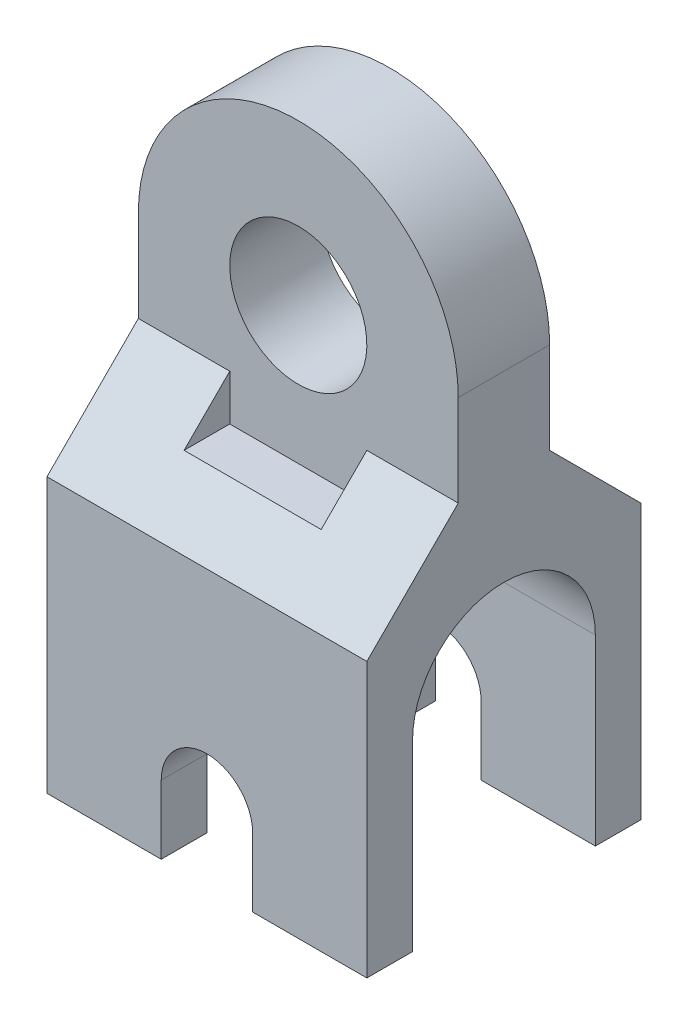
ISO-10303-21;
HEADER;
FILE_DESCRIPTION(('STEP AP214'),'2;1');
FILE_NAME('part.step','',(''),(''),'','','');
FILE_SCHEMA(('AUTOMOTIVE_DESIGN { 1 0 10303 214 1 1 1 1 }'));
ENDSEC;
DATA;
#1=APPLICATION_CONTEXT('core data for automotive mechanical design processes');
#2=APPLICATION_PROTOCOL_DEFINITION('international standard','automotive_design',2000,#1);
#3=PRODUCT_CONTEXT('',#1,'mechanical');
#4=PRODUCT('Part','Part','',(#3));
#5=PRODUCT_RELATED_PRODUCT_CATEGORY('part','',(#4));
#6=PRODUCT_DEFINITION_FORMATION('','',#4);
#7=PRODUCT_DEFINITION_CONTEXT('part definition',#1,'design');
#8=PRODUCT_DEFINITION('design','',#6,#7);
#9=PRODUCT_DEFINITION_SHAPE('','',#8);
#10=(LENGTH_UNIT() NAMED_UNIT(*) SI_UNIT(.MILLI.,.METRE.));
#11=(NAMED_UNIT(*) PLANE_ANGLE_UNIT() SI_UNIT($,.RADIAN.));
#12=(NAMED_UNIT(*) SI_UNIT($,.STERADIAN.) SOLID_ANGLE_UNIT());
#13=UNCERTAINTY_MEASURE_WITH_UNIT(LENGTH_MEASURE(1.E-05),#10,'distance_accuracy_value','');
#14=(GEOMETRIC_REPRESENTATION_CONTEXT(3) GLOBAL_UNCERTAINTY_ASSIGNED_CONTEXT((#13)) GLOBAL_UNIT_ASSIGNED_CONTEXT((#10,
#11,#12)) REPRESENTATION_CONTEXT('',''));
#15=CARTESIAN_POINT('',(0.,0.,0.));
#16=DIRECTION('',(0.,0.,1.));
#17=DIRECTION('',(1.,0.,0.));
#18=AXIS2_PLACEMENT_3D('',#15,#16,#17);
#19=CARTESIAN_POINT('',(35.,0.,30.));
#20=DIRECTION('',(0.,-0.707106781186548,-0.707106781186548));
#21=DIRECTION('',(0.,0.707106781186548,-0.707106781186548));
#22=AXIS2_PLACEMENT_3D('',#19,#20,#21);
#23=PLANE('',#22);
#24=DIRECTION('',(0.,-0.707106781186548,0.707106781186548));
#25=VECTOR('',#24,1.);
#26=CARTESIAN_POINT('',(-15.,0.,30.));
#27=LINE('',#26,#25);
#28=CARTESIAN_POINT('',(-15.,20.,10.));
#29=VERTEX_POINT('',#28);
#30=CARTESIAN_POINT('',(-15.,10.,20.));
#31=VERTEX_POINT('',#30);
#32=EDGE_CURVE('E11',#29,#31,#27,.T.);
#33=ORIENTED_EDGE('',*,*,#32,.F.);
#34=DIRECTION('',(-1.,0.,0.));
#35=VECTOR('',#34,1.);
#36=CARTESIAN_POINT('',(35.,20.,10.));
#37=LINE('',#36,#35);
#38=CARTESIAN_POINT('',(-35.,20.,10.));
#39=VERTEX_POINT('',#38);
#40=EDGE_CURVE('E367',#29,#39,#37,.T.);
#41=ORIENTED_EDGE('',*,*,#40,.T.);
#42=DIRECTION('',(0.,-0.707106781186548,0.707106781186548));
#43=VECTOR('',#42,1.);
#44=CARTESIAN_POINT('',(-35.,0.,30.));
#45=LINE('',#44,#43);
#46=CARTESIAN_POINT('',(-35.,0.,30.));
#47=VERTEX_POINT('',#46);
#48=EDGE_CURVE('E316',#39,#47,#45,.T.);
#49=ORIENTED_EDGE('',*,*,#48,.T.);
#50=DIRECTION('',(-1.,0.,0.));
#51=VECTOR('',#50,1.);
#52=CARTESIAN_POINT('',(35.,0.,30.));
#53=LINE('',#52,#51);
#54=CARTESIAN_POINT('',(35.,0.,30.));
#55=VERTEX_POINT('',#54);
#56=EDGE_CURVE('E337',#55,#47,#53,.T.);
#57=ORIENTED_EDGE('',*,*,#56,.F.);
#58=DIRECTION('',(0.,-0.707106781186548,0.707106781186548));
#59=VECTOR('',#58,1.);
#60=CARTESIAN_POINT('',(35.,0.,30.));
#61=LINE('',#60,#59);
#62=CARTESIAN_POINT('',(35.,20.,10.));
#63=VERTEX_POINT('',#62);
#64=EDGE_CURVE('E338',#63,#55,#61,.T.);
#65=ORIENTED_EDGE('',*,*,#64,.F.);
#66=CARTESIAN_POINT('',(15.,20.,10.));
#67=VERTEX_POINT('',#66);
#68=EDGE_CURVE('E371',#63,#67,#37,.T.);
#69=ORIENTED_EDGE('',*,*,#68,.T.);
#70=DIRECTION('',(0.,0.707106781186548,-0.707106781186548));
#71=VECTOR('',#70,1.);
#72=CARTESIAN_POINT('',(15.,0.,30.));
#73=LINE('',#72,#71);
#74=CARTESIAN_POINT('',(15.,10.,20.));
#75=VERTEX_POINT('',#74);
#76=EDGE_CURVE('E47',#75,#67,#73,.T.);
#77=ORIENTED_EDGE('',*,*,#76,.F.);
#78=DIRECTION('',(-1.,0.,0.));
#79=VECTOR('',#78,1.);
#80=CARTESIAN_POINT('',(-15.,10.,20.));
#81=LINE('',#80,#79);
#82=EDGE_CURVE('E228',#75,#31,#81,.T.);
#83=ORIENTED_EDGE('',*,*,#82,.T.);
#84=EDGE_LOOP('',(#33,#41,#49,#57,#65,#69,#77,#83));
#85=FACE_BOUND('',#84,.T.);
#86=ADVANCED_FACE('F41',(#85),#23,.F.);
#87=CARTESIAN_POINT('',(35.,-60.,30.));
#88=DIRECTION('',(0.,1.,0.));
#89=DIRECTION('',(0.,0.,1.));
#90=AXIS2_PLACEMENT_3D('',#87,#88,#89);
#91=PLANE('',#90);
#92=DIRECTION('',(-1.,0.,0.));
#93=VECTOR('',#92,1.);
#94=CARTESIAN_POINT('',(35.,-60.,20.));
#95=LINE('',#94,#93);
#96=CARTESIAN_POINT('',(-10.,-60.,20.));
#97=VERTEX_POINT('',#96);
#98=CARTESIAN_POINT('',(-35.,-60.,20.));
#99=VERTEX_POINT('',#98);
#100=EDGE_CURVE('E395',#97,#99,#95,.T.);
#101=ORIENTED_EDGE('',*,*,#100,.F.);
#102=DIRECTION('',(0.,0.,-1.));
#103=VECTOR('',#102,1.);
#104=CARTESIAN_POINT('',(-10.,-60.,30.0000000000001));
#105=LINE('',#104,#103);
#106=CARTESIAN_POINT('',(-10.,-60.,30.0000000000001));
#107=VERTEX_POINT('',#106);
#108=EDGE_CURVE('E274',#107,#97,#105,.T.);
#109=ORIENTED_EDGE('',*,*,#108,.F.);
#110=DIRECTION('',(-1.,0.,0.));
#111=VECTOR('',#110,1.);
#112=CARTESIAN_POINT('',(35.,-60.,30.));
#113=LINE('',#112,#111);
#114=CARTESIAN_POINT('',(-35.,-60.,30.));
#115=VERTEX_POINT('',#114);
#116=EDGE_CURVE('E400',#107,#115,#113,.T.);
#117=ORIENTED_EDGE('',*,*,#116,.T.);
#118=DIRECTION('',(0.,0.,-1.));
#119=VECTOR('',#118,1.);
#120=CARTESIAN_POINT('',(-35.,-60.,30.));
#121=LINE('',#120,#119);
#122=EDGE_CURVE('E342',#115,#99,#121,.T.);
#123=ORIENTED_EDGE('',*,*,#122,.T.);
#124=EDGE_LOOP('',(#101,#109,#117,#123));
#125=FACE_BOUND('',#124,.T.);
#126=ADVANCED_FACE('F440',(#125),#91,.F.);
#127=CARTESIAN_POINT('',(35.,-60.,-20.));
#128=DIRECTION('',(0.,1.,0.));
#129=DIRECTION('',(0.,0.,1.));
#130=AXIS2_PLACEMENT_3D('',#127,#128,#129);
#131=PLANE('',#130);
#132=DIRECTION('',(-1.,0.,0.));
#133=VECTOR('',#132,1.);
#134=CARTESIAN_POINT('',(35.,-60.,-30.));
#135=LINE('',#134,#133);
#136=CARTESIAN_POINT('',(-10.,-60.,-30.));
#137=VERTEX_POINT('',#136);
#138=CARTESIAN_POINT('',(-35.,-60.,-30.));
#139=VERTEX_POINT('',#138);
#140=EDGE_CURVE('E379',#137,#139,#135,.T.);
#141=ORIENTED_EDGE('',*,*,#140,.F.);
#142=CARTESIAN_POINT('',(-10.,-60.,-20.));
#143=VERTEX_POINT('',#142);
#144=EDGE_CURVE('E280',#143,#137,#105,.T.);
#145=ORIENTED_EDGE('',*,*,#144,.F.);
#146=DIRECTION('',(-1.,0.,0.));
#147=VECTOR('',#146,1.);
#148=CARTESIAN_POINT('',(35.,-60.,-20.));
#149=LINE('',#148,#147);
#150=CARTESIAN_POINT('',(-35.,-60.,-20.));
#151=VERTEX_POINT('',#150);
#152=EDGE_CURVE('E383',#143,#151,#149,.T.);
#153=ORIENTED_EDGE('',*,*,#152,.T.);
#154=DIRECTION('',(0.,0.,-1.));
#155=VECTOR('',#154,1.);
#156=CARTESIAN_POINT('',(-35.,-60.,-20.));
#157=LINE('',#156,#155);
#158=EDGE_CURVE('E353',#151,#139,#157,.T.);
#159=ORIENTED_EDGE('',*,*,#158,.T.);
#160=EDGE_LOOP('',(#141,#145,#153,#159));
#161=FACE_BOUND('',#160,.T.);
#162=ADVANCED_FACE('F473',(#161),#131,.F.);
#163=CARTESIAN_POINT('',(35.,0.,30.));
#164=DIRECTION('',(0.,0.,-1.));
#165=DIRECTION('',(0.,1.,0.));
#166=AXIS2_PLACEMENT_3D('',#163,#164,#165);
#167=PLANE('',#166);
#168=ORIENTED_EDGE('',*,*,#116,.F.);
#169=DIRECTION('',(0.,1.,0.));
#170=VECTOR('',#169,1.);
#171=CARTESIAN_POINT('',(-10.,-45.,30.0000000000001));
#172=LINE('',#171,#170);
#173=CARTESIAN_POINT('',(-10.,-45.,30.0000000000001));
#174=VERTEX_POINT('',#173);
#175=EDGE_CURVE('E266',#107,#174,#172,.T.);
#176=ORIENTED_EDGE('',*,*,#175,.T.);
#177=CARTESIAN_POINT('',(0.,-45.,30.0000000000001));
#178=DIRECTION('',(0.,0.,-1.));
#179=DIRECTION('',(0.,1.,0.));
#180=AXIS2_PLACEMENT_3D('',#177,#178,#179);
#181=CIRCLE('',#180,10.);
#182=CARTESIAN_POINT('',(10.,-45.,30.0000000000001));
#183=VERTEX_POINT('',#182);
#184=EDGE_CURVE('E257',#174,#183,#181,.T.);
#185=ORIENTED_EDGE('',*,*,#184,.T.);
#186=DIRECTION('',(0.,-1.,0.));
#187=VECTOR('',#186,1.);
#188=CARTESIAN_POINT('',(10.,-45.,30.0000000000001));
#189=LINE('',#188,#187);
#190=CARTESIAN_POINT('',(10.,-60.,30.0000000000001));
#191=VERTEX_POINT('',#190);
#192=EDGE_CURVE('E263',#183,#191,#189,.T.);
#193=ORIENTED_EDGE('',*,*,#192,.T.);
#194=CARTESIAN_POINT('',(35.,-60.,30.));
#195=VERTEX_POINT('',#194);
#196=EDGE_CURVE('E396',#195,#191,#113,.T.);
#197=ORIENTED_EDGE('',*,*,#196,.F.);
#198=DIRECTION('',(0.,-1.,0.));
#199=VECTOR('',#198,1.);
#200=CARTESIAN_POINT('',(35.,0.,30.));
#201=LINE('',#200,#199);
#202=EDGE_CURVE('E315',#55,#195,#201,.T.);
#203=ORIENTED_EDGE('',*,*,#202,.F.);
#204=ORIENTED_EDGE('',*,*,#56,.T.);
#205=DIRECTION('',(0.,-1.,0.));
#206=VECTOR('',#205,1.);
#207=CARTESIAN_POINT('',(-35.,0.,30.));
#208=LINE('',#207,#206);
#209=EDGE_CURVE('E310',#47,#115,#208,.T.);
#210=ORIENTED_EDGE('',*,*,#209,.T.);
#211=EDGE_LOOP('',(#168,#176,#185,#193,#197,#203,#204,#210));
#212=FACE_BOUND('',#211,.T.);
#213=ADVANCED_FACE('F43',(#212),#167,.F.);
#214=ORIENTED_EDGE('',*,*,#196,.T.);
#215=DIRECTION('',(0.,0.,-1.));
#216=VECTOR('',#215,1.);
#217=CARTESIAN_POINT('',(10.,-60.,30.0000000000001));
#218=LINE('',#217,#216);
#219=CARTESIAN_POINT('',(10.,-60.,20.));
#220=VERTEX_POINT('',#219);
#221=EDGE_CURVE('E279',#191,#220,#218,.T.);
#222=ORIENTED_EDGE('',*,*,#221,.T.);
#223=CARTESIAN_POINT('',(35.,-60.,20.));
#224=VERTEX_POINT('',#223);
#225=EDGE_CURVE('E391',#224,#220,#95,.T.);
#226=ORIENTED_EDGE('',*,*,#225,.F.);
#227=DIRECTION('',(0.,0.,-1.));
#228=VECTOR('',#227,1.);
#229=CARTESIAN_POINT('',(35.,-60.,30.));
#230=LINE('',#229,#228);
#231=EDGE_CURVE('E312',#195,#224,#230,.T.);
#232=ORIENTED_EDGE('',*,*,#231,.F.);
#233=EDGE_LOOP('',(#214,#222,#226,#232));
#234=FACE_BOUND('',#233,.T.);
#235=ADVANCED_FACE('F450',(#234),#91,.F.);
#236=CARTESIAN_POINT('',(35.,-60.,20.));
#237=DIRECTION('',(0.,0.,1.));
#238=DIRECTION('',(0.,-1.,0.));
#239=AXIS2_PLACEMENT_3D('',#236,#237,#238);
#240=PLANE('',#239);
#241=CARTESIAN_POINT('',(0.,-45.,20.));
#242=DIRECTION('',(0.,0.,1.));
#243=DIRECTION('',(0.,-1.,0.));
#244=AXIS2_PLACEMENT_3D('',#241,#242,#243);
#245=CIRCLE('',#244,10.);
#246=CARTESIAN_POINT('',(10.,-45.,20.));
#247=VERTEX_POINT('',#246);
#248=CARTESIAN_POINT('',(-10.,-45.,20.));
#249=VERTEX_POINT('',#248);
#250=EDGE_CURVE('E304',#247,#249,#245,.T.);
#251=ORIENTED_EDGE('',*,*,#250,.T.);
#252=DIRECTION('',(0.,-1.,0.));
#253=VECTOR('',#252,1.);
#254=CARTESIAN_POINT('',(-10.,-60.,20.));
#255=LINE('',#254,#253);
#256=EDGE_CURVE('E298',#249,#97,#255,.T.);
#257=ORIENTED_EDGE('',*,*,#256,.T.);
#258=ORIENTED_EDGE('',*,*,#100,.T.);
#259=DIRECTION('',(0.,1.,0.));
#260=VECTOR('',#259,1.);
#261=CARTESIAN_POINT('',(-35.,-60.,20.));
#262=LINE('',#261,#260);
#263=CARTESIAN_POINT('',(-35.,-20.,20.));
#264=VERTEX_POINT('',#263);
#265=EDGE_CURVE('E341',#99,#264,#262,.T.);
#266=ORIENTED_EDGE('',*,*,#265,.T.);
#267=DIRECTION('',(-1.,0.,0.));
#268=VECTOR('',#267,1.);
#269=CARTESIAN_POINT('',(35.,-20.,20.));
#270=LINE('',#269,#268);
#271=CARTESIAN_POINT('',(35.,-20.,20.));
#272=VERTEX_POINT('',#271);
#273=EDGE_CURVE('E393',#272,#264,#270,.T.);
#274=ORIENTED_EDGE('',*,*,#273,.F.);
#275=DIRECTION('',(0.,1.,0.));
#276=VECTOR('',#275,1.);
#277=CARTESIAN_POINT('',(35.,-60.,20.));
#278=LINE('',#277,#276);
#279=EDGE_CURVE('E318',#224,#272,#278,.T.);
#280=ORIENTED_EDGE('',*,*,#279,.F.);
#281=ORIENTED_EDGE('',*,*,#225,.T.);
#282=DIRECTION('',(0.,1.,0.));
#283=VECTOR('',#282,1.);
#284=CARTESIAN_POINT('',(10.,-60.,20.));
#285=LINE('',#284,#283);
#286=EDGE_CURVE('E288',#220,#247,#285,.T.);
#287=ORIENTED_EDGE('',*,*,#286,.T.);
#288=EDGE_LOOP('',(#251,#257,#258,#266,#274,#280,#281,#287));
#289=FACE_BOUND('',#288,.T.);
#290=ADVANCED_FACE('F493',(#289),#240,.F.);
#291=CARTESIAN_POINT('',(35.,-20.,0.));
#292=DIRECTION('',(-1.,0.,0.));
#293=DIRECTION('',(0.,0.,1.));
#294=AXIS2_PLACEMENT_3D('',#291,#292,#293);
#295=CYLINDRICAL_SURFACE('',#294,20.);
#296=CARTESIAN_POINT('',(-35.,-20.,0.));
#297=DIRECTION('',(-1.,0.,0.));
#298=DIRECTION('',(0.,0.,1.));
#299=AXIS2_PLACEMENT_3D('',#296,#297,#298);
#300=CIRCLE('',#299,20.);
#301=CARTESIAN_POINT('',(-35.,-20.,-20.));
#302=VERTEX_POINT('',#301);
#303=EDGE_CURVE('E347',#264,#302,#300,.T.);
#304=ORIENTED_EDGE('',*,*,#303,.T.);
#305=DIRECTION('',(-1.,0.,0.));
#306=VECTOR('',#305,1.);
#307=CARTESIAN_POINT('',(35.,-20.,-20.));
#308=LINE('',#307,#306);
#309=CARTESIAN_POINT('',(35.,-20.,-20.));
#310=VERTEX_POINT('',#309);
#311=EDGE_CURVE('E389',#310,#302,#308,.T.);
#312=ORIENTED_EDGE('',*,*,#311,.F.);
#313=CARTESIAN_POINT('',(35.,-20.,0.));
#314=DIRECTION('',(-1.,0.,0.));
#315=DIRECTION('',(0.,0.,1.));
#316=AXIS2_PLACEMENT_3D('',#313,#314,#315);
#317=CIRCLE('',#316,20.);
#318=EDGE_CURVE('E319',#272,#310,#317,.T.);
#319=ORIENTED_EDGE('',*,*,#318,.F.);
#320=ORIENTED_EDGE('',*,*,#273,.T.);
#321=EDGE_LOOP('',(#304,#312,#319,#320));
#322=FACE_BOUND('',#321,.T.);
#323=ADVANCED_FACE('F491',(#322),#295,.F.);
#324=CARTESIAN_POINT('',(35.,-20.,-20.));
#325=DIRECTION('',(0.,0.,-1.));
#326=DIRECTION('',(-1.,0.,0.));
#327=AXIS2_PLACEMENT_3D('',#324,#325,#326);
#328=PLANE('',#327);
#329=ORIENTED_EDGE('',*,*,#152,.F.);
#330=DIRECTION('',(0.,1.,0.));
#331=VECTOR('',#330,1.);
#332=CARTESIAN_POINT('',(-10.,-20.,-20.));
#333=LINE('',#332,#331);
#334=CARTESIAN_POINT('',(-10.,-45.,-20.));
#335=VERTEX_POINT('',#334);
#336=EDGE_CURVE('E291',#143,#335,#333,.T.);
#337=ORIENTED_EDGE('',*,*,#336,.T.);
#338=CARTESIAN_POINT('',(0.,-45.,-20.));
#339=DIRECTION('',(0.,0.,-1.));
#340=DIRECTION('',(-1.,0.,0.));
#341=AXIS2_PLACEMENT_3D('',#338,#339,#340);
#342=CIRCLE('',#341,10.);
#343=CARTESIAN_POINT('',(10.,-45.,-20.));
#344=VERTEX_POINT('',#343);
#345=EDGE_CURVE('E300',#335,#344,#342,.T.);
#346=ORIENTED_EDGE('',*,*,#345,.T.);
#347=DIRECTION('',(0.,-1.,0.));
#348=VECTOR('',#347,1.);
#349=CARTESIAN_POINT('',(10.,-20.,-20.));
#350=LINE('',#349,#348);
#351=CARTESIAN_POINT('',(10.,-60.,-20.));
#352=VERTEX_POINT('',#351);
#353=EDGE_CURVE('E289',#344,#352,#350,.T.);
#354=ORIENTED_EDGE('',*,*,#353,.T.);
#355=CARTESIAN_POINT('',(35.,-60.,-20.));
#356=VERTEX_POINT('',#355);
#357=EDGE_CURVE('E384',#356,#352,#149,.T.);
#358=ORIENTED_EDGE('',*,*,#357,.F.);
#359=DIRECTION('',(0.,-1.,0.));
#360=VECTOR('',#359,1.);
#361=CARTESIAN_POINT('',(35.,-20.,-20.));
#362=LINE('',#361,#360);
#363=EDGE_CURVE('E325',#310,#356,#362,.T.);
#364=ORIENTED_EDGE('',*,*,#363,.F.);
#365=ORIENTED_EDGE('',*,*,#311,.T.);
#366=DIRECTION('',(0.,-1.,0.));
#367=VECTOR('',#366,1.);
#368=CARTESIAN_POINT('',(-35.,-20.,-20.));
#369=LINE('',#368,#367);
#370=EDGE_CURVE('E346',#302,#151,#369,.T.);
#371=ORIENTED_EDGE('',*,*,#370,.T.);
#372=EDGE_LOOP('',(#329,#337,#346,#354,#358,#364,#365,#371));
#373=FACE_BOUND('',#372,.T.);
#374=ADVANCED_FACE('F490',(#373),#328,.F.);
#375=ORIENTED_EDGE('',*,*,#357,.T.);
#376=CARTESIAN_POINT('',(10.,-60.,-30.));
#377=VERTEX_POINT('',#376);
#378=EDGE_CURVE('E283',#352,#377,#218,.T.);
#379=ORIENTED_EDGE('',*,*,#378,.T.);
#380=CARTESIAN_POINT('',(35.,-60.,-30.));
#381=VERTEX_POINT('',#380);
#382=EDGE_CURVE('E381',#381,#377,#135,.T.);
#383=ORIENTED_EDGE('',*,*,#382,.F.);
#384=DIRECTION('',(0.,0.,-1.));
#385=VECTOR('',#384,1.);
#386=CARTESIAN_POINT('',(35.,-60.,-20.));
#387=LINE('',#386,#385);
#388=EDGE_CURVE('E322',#356,#381,#387,.T.);
#389=ORIENTED_EDGE('',*,*,#388,.F.);
#390=EDGE_LOOP('',(#375,#379,#383,#389));
#391=FACE_BOUND('',#390,.T.);
#392=ADVANCED_FACE('F483',(#391),#131,.F.);
#393=CARTESIAN_POINT('',(35.,0.,-30.));
#394=DIRECTION('',(0.,0.,1.));
#395=DIRECTION('',(0.,-1.,0.));
#396=AXIS2_PLACEMENT_3D('',#393,#394,#395);
#397=PLANE('',#396);
#398=CARTESIAN_POINT('',(0.,-45.,-30.));
#399=DIRECTION('',(0.,0.,-1.));
#400=DIRECTION('',(0.,1.,0.));
#401=AXIS2_PLACEMENT_3D('',#398,#399,#400);
#402=CIRCLE('',#401,10.);
#403=CARTESIAN_POINT('',(-10.,-45.,-30.));
#404=VERTEX_POINT('',#403);
#405=CARTESIAN_POINT('',(10.,-45.,-30.));
#406=VERTEX_POINT('',#405);
#407=EDGE_CURVE('E252',#404,#406,#402,.T.);
#408=ORIENTED_EDGE('',*,*,#407,.F.);
#409=DIRECTION('',(0.,1.,0.));
#410=VECTOR('',#409,1.);
#411=CARTESIAN_POINT('',(-10.,-45.,-30.));
#412=LINE('',#411,#410);
#413=EDGE_CURVE('E260',#137,#404,#412,.T.);
#414=ORIENTED_EDGE('',*,*,#413,.F.);
#415=ORIENTED_EDGE('',*,*,#140,.T.);
#416=DIRECTION('',(0.,1.,0.));
#417=VECTOR('',#416,1.);
#418=CARTESIAN_POINT('',(-35.,0.,-30.));
#419=LINE('',#418,#417);
#420=CARTESIAN_POINT('',(-35.,0.,-30.));
#421=VERTEX_POINT('',#420);
#422=EDGE_CURVE('E355',#139,#421,#419,.T.);
#423=ORIENTED_EDGE('',*,*,#422,.T.);
#424=DIRECTION('',(-1.,0.,0.));
#425=VECTOR('',#424,1.);
#426=CARTESIAN_POINT('',(35.,0.,-30.));
#427=LINE('',#426,#425);
#428=CARTESIAN_POINT('',(35.,0.,-30.));
#429=VERTEX_POINT('',#428);
#430=EDGE_CURVE('E380',#429,#421,#427,.T.);
#431=ORIENTED_EDGE('',*,*,#430,.F.);
#432=DIRECTION('',(0.,1.,0.));
#433=VECTOR('',#432,1.);
#434=CARTESIAN_POINT('',(35.,0.,-30.));
#435=LINE('',#434,#433);
#436=EDGE_CURVE('E326',#381,#429,#435,.T.);
#437=ORIENTED_EDGE('',*,*,#436,.F.);
#438=ORIENTED_EDGE('',*,*,#382,.T.);
#439=DIRECTION('',(0.,-1.,0.));
#440=VECTOR('',#439,1.);
#441=CARTESIAN_POINT('',(10.,-45.,-30.));
#442=LINE('',#441,#440);
#443=EDGE_CURVE('E254',#406,#377,#442,.T.);
#444=ORIENTED_EDGE('',*,*,#443,.F.);
#445=EDGE_LOOP('',(#408,#414,#415,#423,#431,#437,#438,#444));
#446=FACE_BOUND('',#445,.T.);
#447=ADVANCED_FACE('F479',(#446),#397,.F.);
#448=CARTESIAN_POINT('',(35.,20.,-9.99999999999999));
#449=DIRECTION('',(0.,-0.707106781186548,0.707106781186547));
#450=DIRECTION('',(0.,-0.707106781186547,-0.707106781186548));
#451=AXIS2_PLACEMENT_3D('',#448,#449,#450);
#452=PLANE('',#451);
#453=DIRECTION('',(-1.,0.,0.));
#454=VECTOR('',#453,1.);
#455=CARTESIAN_POINT('',(35.,20.,-9.99999999999999));
#456=LINE('',#455,#454);
#457=CARTESIAN_POINT('',(-15.,20.,-9.99999999999999));
#458=VERTEX_POINT('',#457);
#459=CARTESIAN_POINT('',(-35.,20.,-9.99999999999999));
#460=VERTEX_POINT('',#459);
#461=EDGE_CURVE('E373',#458,#460,#456,.T.);
#462=ORIENTED_EDGE('',*,*,#461,.F.);
#463=DIRECTION('',(0.,-0.707106781186547,-0.707106781186548));
#464=VECTOR('',#463,1.);
#465=CARTESIAN_POINT('',(-15.,20.,-9.99999999999999));
#466=LINE('',#465,#464);
#467=CARTESIAN_POINT('',(-15.,10.,-20.));
#468=VERTEX_POINT('',#467);
#469=EDGE_CURVE('E409',#458,#468,#466,.T.);
#470=ORIENTED_EDGE('',*,*,#469,.T.);
#471=DIRECTION('',(-1.,0.,0.));
#472=VECTOR('',#471,1.);
#473=CARTESIAN_POINT('',(-15.,10.,-20.));
#474=LINE('',#473,#472);
#475=CARTESIAN_POINT('',(15.,10.,-20.));
#476=VERTEX_POINT('',#475);
#477=EDGE_CURVE('E249',#476,#468,#474,.T.);
#478=ORIENTED_EDGE('',*,*,#477,.F.);
#479=DIRECTION('',(0.,0.707106781186547,0.707106781186548));
#480=VECTOR('',#479,1.);
#481=CARTESIAN_POINT('',(15.,20.,-9.99999999999999));
#482=LINE('',#481,#480);
#483=CARTESIAN_POINT('',(15.,20.,-10.));
#484=VERTEX_POINT('',#483);
#485=EDGE_CURVE('E405',#476,#484,#482,.T.);
#486=ORIENTED_EDGE('',*,*,#485,.T.);
#487=CARTESIAN_POINT('',(35.,20.,-9.99999999999999));
#488=VERTEX_POINT('',#487);
#489=EDGE_CURVE('E372',#488,#484,#456,.T.);
#490=ORIENTED_EDGE('',*,*,#489,.F.);
#491=DIRECTION('',(0.,0.707106781186547,0.707106781186548));
#492=VECTOR('',#491,1.);
#493=CARTESIAN_POINT('',(35.,20.,-9.99999999999999));
#494=LINE('',#493,#492);
#495=EDGE_CURVE('E327',#429,#488,#494,.T.);
#496=ORIENTED_EDGE('',*,*,#495,.F.);
#497=ORIENTED_EDGE('',*,*,#430,.T.);
#498=DIRECTION('',(0.,0.707106781186547,0.707106781186548));
#499=VECTOR('',#498,1.);
#500=CARTESIAN_POINT('',(-35.,20.,-9.99999999999999));
#501=LINE('',#500,#499);
#502=EDGE_CURVE('E357',#421,#460,#501,.T.);
#503=ORIENTED_EDGE('',*,*,#502,.T.);
#504=EDGE_LOOP('',(#462,#470,#478,#486,#490,#496,#497,#503));
#505=FACE_BOUND('',#504,.T.);
#506=ADVANCED_FACE('F474',(#505),#452,.F.);
#507=CARTESIAN_POINT('',(35.,20.,-9.99999999999999));
#508=DIRECTION('',(0.,0.,1.));
#509=DIRECTION('',(0.,-1.,0.));
#510=AXIS2_PLACEMENT_3D('',#507,#508,#509);
#511=PLANE('',#510);
#512=CARTESIAN_POINT('',(0.,40.,-10.));
#513=DIRECTION('',(0.,0.,1.));
#514=DIRECTION('',(0.,-1.,0.));
#515=AXIS2_PLACEMENT_3D('',#512,#513,#514);
#516=CIRCLE('',#515,15.);
#517=CARTESIAN_POINT('',(0.,25.,-10.));
#518=VERTEX_POINT('',#517);
#519=EDGE_CURVE('E285',#518,#518,#516,.T.);
#520=ORIENTED_EDGE('',*,*,#519,.T.);
#521=EDGE_LOOP('',(#520));
#522=FACE_BOUND('',#521,.T.);
#523=DIRECTION('',(0.,1.,0.));
#524=VECTOR('',#523,1.);
#525=CARTESIAN_POINT('',(-35.,20.,-9.99999999999999));
#526=LINE('',#525,#524);
#527=CARTESIAN_POINT('',(-35.,40.,-10.));
#528=VERTEX_POINT('',#527);
#529=EDGE_CURVE('E356',#460,#528,#526,.T.);
#530=ORIENTED_EDGE('',*,*,#529,.T.);
#531=CARTESIAN_POINT('',(0.,40.,-10.));
#532=DIRECTION('',(0.,0.,-1.));
#533=DIRECTION('',(0.,-1.,0.));
#534=AXIS2_PLACEMENT_3D('',#531,#532,#533);
#535=CIRCLE('',#534,35.);
#536=CARTESIAN_POINT('',(35.,40.,-10.));
#537=VERTEX_POINT('',#536);
#538=EDGE_CURVE('E303',#528,#537,#535,.T.);
#539=ORIENTED_EDGE('',*,*,#538,.T.);
#540=DIRECTION('',(0.,1.,0.));
#541=VECTOR('',#540,1.);
#542=CARTESIAN_POINT('',(35.,20.,-9.99999999999999));
#543=LINE('',#542,#541);
#544=EDGE_CURVE('E329',#488,#537,#543,.T.);
#545=ORIENTED_EDGE('',*,*,#544,.F.);
#546=ORIENTED_EDGE('',*,*,#489,.T.);
#547=DIRECTION('',(0.,1.,0.));
#548=VECTOR('',#547,1.);
#549=CARTESIAN_POINT('',(15.,10.,-10.));
#550=LINE('',#549,#548);
#551=CARTESIAN_POINT('',(15.,10.,-10.));
#552=VERTEX_POINT('',#551);
#553=EDGE_CURVE('E248',#552,#484,#550,.T.);
#554=ORIENTED_EDGE('',*,*,#553,.F.);
#555=DIRECTION('',(1.,0.,0.));
#556=VECTOR('',#555,1.);
#557=CARTESIAN_POINT('',(-15.,10.,-10.));
#558=LINE('',#557,#556);
#559=CARTESIAN_POINT('',(-15.,10.,-10.));
#560=VERTEX_POINT('',#559);
#561=EDGE_CURVE('E243',#560,#552,#558,.T.);
#562=ORIENTED_EDGE('',*,*,#561,.F.);
#563=DIRECTION('',(0.,1.,0.));
#564=VECTOR('',#563,1.);
#565=CARTESIAN_POINT('',(-15.,10.,-10.));
#566=LINE('',#565,#564);
#567=EDGE_CURVE('E65',#560,#458,#566,.T.);
#568=ORIENTED_EDGE('',*,*,#567,.T.);
#569=ORIENTED_EDGE('',*,*,#461,.T.);
#570=EDGE_LOOP('',(#530,#539,#545,#546,#554,#562,#568,#569));
#571=FACE_BOUND('',#570,.T.);
#572=ADVANCED_FACE('F463',(#522,#571),#511,.F.);
#573=CARTESIAN_POINT('',(35.,20.,10.));
#574=DIRECTION('',(0.,0.,-1.));
#575=DIRECTION('',(0.,1.,0.));
#576=AXIS2_PLACEMENT_3D('',#573,#574,#575);
#577=PLANE('',#576);
#578=CARTESIAN_POINT('',(0.,40.,10.));
#579=DIRECTION('',(0.,0.,-1.));
#580=DIRECTION('',(0.,1.,0.));
#581=AXIS2_PLACEMENT_3D('',#578,#579,#580);
#582=CIRCLE('',#581,15.);
#583=CARTESIAN_POINT('',(0.,55.,10.));
#584=VERTEX_POINT('',#583);
#585=EDGE_CURVE('E272',#584,#584,#582,.T.);
#586=ORIENTED_EDGE('',*,*,#585,.T.);
#587=EDGE_LOOP('',(#586));
#588=FACE_BOUND('',#587,.T.);
#589=DIRECTION('',(0.,-1.,0.));
#590=VECTOR('',#589,1.);
#591=CARTESIAN_POINT('',(-35.,20.,10.));
#592=LINE('',#591,#590);
#593=CARTESIAN_POINT('',(-35.,40.,10.));
#594=VERTEX_POINT('',#593);
#595=EDGE_CURVE('E365',#594,#39,#592,.T.);
#596=ORIENTED_EDGE('',*,*,#595,.T.);
#597=ORIENTED_EDGE('',*,*,#40,.F.);
#598=DIRECTION('',(0.,1.,0.));
#599=VECTOR('',#598,1.);
#600=CARTESIAN_POINT('',(-15.,10.,10.));
#601=LINE('',#600,#599);
#602=CARTESIAN_POINT('',(-15.,10.,10.));
#603=VERTEX_POINT('',#602);
#604=EDGE_CURVE('E217',#603,#29,#601,.T.);
#605=ORIENTED_EDGE('',*,*,#604,.F.);
#606=DIRECTION('',(1.,0.,0.));
#607=VECTOR('',#606,1.);
#608=CARTESIAN_POINT('',(-15.,10.,10.));
#609=LINE('',#608,#607);
#610=CARTESIAN_POINT('',(15.,10.,10.));
#611=VERTEX_POINT('',#610);
#612=EDGE_CURVE('E227',#603,#611,#609,.T.);
#613=ORIENTED_EDGE('',*,*,#612,.T.);
#614=DIRECTION('',(0.,1.,0.));
#615=VECTOR('',#614,1.);
#616=CARTESIAN_POINT('',(15.,10.,10.));
#617=LINE('',#616,#615);
#618=EDGE_CURVE('E57',#611,#67,#617,.T.);
#619=ORIENTED_EDGE('',*,*,#618,.T.);
#620=ORIENTED_EDGE('',*,*,#68,.F.);
#621=DIRECTION('',(0.,-1.,0.));
#622=VECTOR('',#621,1.);
#623=CARTESIAN_POINT('',(35.,20.,10.));
#624=LINE('',#623,#622);
#625=CARTESIAN_POINT('',(35.,40.,10.));
#626=VERTEX_POINT('',#625);
#627=EDGE_CURVE('E331',#626,#63,#624,.T.);
#628=ORIENTED_EDGE('',*,*,#627,.F.);
#629=CARTESIAN_POINT('',(0.,40.,10.));
#630=DIRECTION('',(0.,0.,-1.));
#631=DIRECTION('',(0.,-1.,0.));
#632=AXIS2_PLACEMENT_3D('',#629,#630,#631);
#633=CIRCLE('',#632,35.);
#634=EDGE_CURVE('E308',#594,#626,#633,.T.);
#635=ORIENTED_EDGE('',*,*,#634,.F.);
#636=EDGE_LOOP('',(#596,#597,#605,#613,#619,#620,#628,#635));
#637=FACE_BOUND('',#636,.T.);
#638=ADVANCED_FACE('F411',(#588,#637),#577,.F.);
#639=CARTESIAN_POINT('',(35.,-20.,0.));
#640=DIRECTION('',(-1.,0.,0.));
#641=DIRECTION('',(0.,0.,1.));
#642=AXIS2_PLACEMENT_3D('',#639,#640,#641);
#643=PLANE('',#642);
#644=ORIENTED_EDGE('',*,*,#202,.T.);
#645=ORIENTED_EDGE('',*,*,#231,.T.);
#646=ORIENTED_EDGE('',*,*,#279,.T.);
#647=ORIENTED_EDGE('',*,*,#318,.T.);
#648=ORIENTED_EDGE('',*,*,#363,.T.);
#649=ORIENTED_EDGE('',*,*,#388,.T.);
#650=ORIENTED_EDGE('',*,*,#436,.T.);
#651=ORIENTED_EDGE('',*,*,#495,.T.);
#652=ORIENTED_EDGE('',*,*,#544,.T.);
#653=DIRECTION('',(0.,0.,1.));
#654=VECTOR('',#653,1.);
#655=CARTESIAN_POINT('',(35.,40.,10.));
#656=LINE('',#655,#654);
#657=EDGE_CURVE('E335',#537,#626,#656,.T.);
#658=ORIENTED_EDGE('',*,*,#657,.T.);
#659=ORIENTED_EDGE('',*,*,#627,.T.);
#660=ORIENTED_EDGE('',*,*,#64,.T.);
#661=EDGE_LOOP('',(#644,#645,#646,#647,#648,#649,#650,#651,#652,#658,#659,#660));
#662=FACE_BOUND('',#661,.T.);
#663=ADVANCED_FACE('F454',(#662),#643,.F.);
#664=CARTESIAN_POINT('',(-35.,-20.,0.));
#665=DIRECTION('',(-1.,0.,0.));
#666=DIRECTION('',(0.,0.,1.));
#667=AXIS2_PLACEMENT_3D('',#664,#665,#666);
#668=PLANE('',#667);
#669=ORIENTED_EDGE('',*,*,#209,.F.);
#670=ORIENTED_EDGE('',*,*,#48,.F.);
#671=ORIENTED_EDGE('',*,*,#595,.F.);
#672=DIRECTION('',(0.,0.,1.));
#673=VECTOR('',#672,1.);
#674=CARTESIAN_POINT('',(-35.,40.,10.));
#675=LINE('',#674,#673);
#676=EDGE_CURVE('E363',#528,#594,#675,.T.);
#677=ORIENTED_EDGE('',*,*,#676,.F.);
#678=ORIENTED_EDGE('',*,*,#529,.F.);
#679=ORIENTED_EDGE('',*,*,#502,.F.);
#680=ORIENTED_EDGE('',*,*,#422,.F.);
#681=ORIENTED_EDGE('',*,*,#158,.F.);
#682=ORIENTED_EDGE('',*,*,#370,.F.);
#683=ORIENTED_EDGE('',*,*,#303,.F.);
#684=ORIENTED_EDGE('',*,*,#265,.F.);
#685=ORIENTED_EDGE('',*,*,#122,.F.);
#686=EDGE_LOOP('',(#669,#670,#671,#677,#678,#679,#680,#681,#682,#683,#684,#685));
#687=FACE_BOUND('',#686,.T.);
#688=ADVANCED_FACE('F422',(#687),#668,.T.);
#689=CARTESIAN_POINT('',(0.,40.,10.));
#690=DIRECTION('',(0.,0.,-1.));
#691=DIRECTION('',(0.,1.,0.));
#692=AXIS2_PLACEMENT_3D('',#689,#690,#691);
#693=CYLINDRICAL_SURFACE('',#692,35.);
#694=ORIENTED_EDGE('',*,*,#538,.F.);
#695=ORIENTED_EDGE('',*,*,#676,.T.);
#696=ORIENTED_EDGE('',*,*,#634,.T.);
#697=ORIENTED_EDGE('',*,*,#657,.F.);
#698=EDGE_LOOP('',(#694,#695,#696,#697));
#699=FACE_BOUND('',#698,.T.);
#700=ADVANCED_FACE('F419',(#699),#693,.T.);
#701=CARTESIAN_POINT('',(0.,40.,30.));
#702=DIRECTION('',(0.,0.,-1.));
#703=DIRECTION('',(0.,1.,0.));
#704=AXIS2_PLACEMENT_3D('',#701,#702,#703);
#705=CYLINDRICAL_SURFACE('',#704,15.);
#706=ORIENTED_EDGE('',*,*,#585,.F.);
#707=EDGE_LOOP('',(#706));
#708=FACE_BOUND('',#707,.T.);
#709=ORIENTED_EDGE('',*,*,#519,.F.);
#710=EDGE_LOOP('',(#709));
#711=FACE_BOUND('',#710,.T.);
#712=ADVANCED_FACE('F546',(#708,#711),#705,.F.);
#713=CARTESIAN_POINT('',(10.,-45.,30.0000000000001));
#714=DIRECTION('',(1.,0.,0.));
#715=DIRECTION('',(0.,1.,0.));
#716=AXIS2_PLACEMENT_3D('',#713,#714,#715);
#717=PLANE('',#716);
#718=DIRECTION('',(0.,0.,-1.));
#719=VECTOR('',#718,1.);
#720=CARTESIAN_POINT('',(10.,-45.,30.0000000000001));
#721=LINE('',#720,#719);
#722=EDGE_CURVE('E267',#344,#406,#721,.T.);
#723=ORIENTED_EDGE('',*,*,#722,.T.);
#724=ORIENTED_EDGE('',*,*,#443,.T.);
#725=ORIENTED_EDGE('',*,*,#378,.F.);
#726=ORIENTED_EDGE('',*,*,#353,.F.);
#727=EDGE_LOOP('',(#723,#724,#725,#726));
#728=FACE_BOUND('',#727,.T.);
#729=ADVANCED_FACE('F531',(#728),#717,.F.);
#730=CARTESIAN_POINT('',(-10.,-45.,30.0000000000001));
#731=DIRECTION('',(-1.,0.,0.));
#732=DIRECTION('',(0.,-1.,0.));
#733=AXIS2_PLACEMENT_3D('',#730,#731,#732);
#734=PLANE('',#733);
#735=ORIENTED_EDGE('',*,*,#144,.T.);
#736=ORIENTED_EDGE('',*,*,#413,.T.);
#737=DIRECTION('',(0.,0.,-1.));
#738=VECTOR('',#737,1.);
#739=CARTESIAN_POINT('',(-10.,-45.,30.0000000000001));
#740=LINE('',#739,#738);
#741=EDGE_CURVE('E273',#335,#404,#740,.T.);
#742=ORIENTED_EDGE('',*,*,#741,.F.);
#743=ORIENTED_EDGE('',*,*,#336,.F.);
#744=EDGE_LOOP('',(#735,#736,#742,#743));
#745=FACE_BOUND('',#744,.T.);
#746=ADVANCED_FACE('F520',(#745),#734,.F.);
#747=CARTESIAN_POINT('',(0.,-45.,30.0000000000001));
#748=DIRECTION('',(0.,0.,-1.));
#749=DIRECTION('',(0.,1.,0.));
#750=AXIS2_PLACEMENT_3D('',#747,#748,#749);
#751=CYLINDRICAL_SURFACE('',#750,10.);
#752=ORIENTED_EDGE('',*,*,#741,.T.);
#753=ORIENTED_EDGE('',*,*,#407,.T.);
#754=ORIENTED_EDGE('',*,*,#722,.F.);
#755=ORIENTED_EDGE('',*,*,#345,.F.);
#756=EDGE_LOOP('',(#752,#753,#754,#755));
#757=FACE_BOUND('',#756,.T.);
#758=ADVANCED_FACE('F536',(#757),#751,.F.);
#759=EDGE_CURVE('E284',#183,#247,#721,.T.);
#760=ORIENTED_EDGE('',*,*,#759,.F.);
#761=ORIENTED_EDGE('',*,*,#184,.F.);
#762=EDGE_CURVE('E269',#174,#249,#740,.T.);
#763=ORIENTED_EDGE('',*,*,#762,.T.);
#764=ORIENTED_EDGE('',*,*,#250,.F.);
#765=EDGE_LOOP('',(#760,#761,#763,#764));
#766=FACE_BOUND('',#765,.T.);
#767=ADVANCED_FACE('F441',(#766),#751,.F.);
#768=ORIENTED_EDGE('',*,*,#762,.F.);
#769=ORIENTED_EDGE('',*,*,#175,.F.);
#770=ORIENTED_EDGE('',*,*,#108,.T.);
#771=ORIENTED_EDGE('',*,*,#256,.F.);
#772=EDGE_LOOP('',(#768,#769,#770,#771));
#773=FACE_BOUND('',#772,.T.);
#774=ADVANCED_FACE('F442',(#773),#734,.F.);
#775=ORIENTED_EDGE('',*,*,#221,.F.);
#776=ORIENTED_EDGE('',*,*,#192,.F.);
#777=ORIENTED_EDGE('',*,*,#759,.T.);
#778=ORIENTED_EDGE('',*,*,#286,.F.);
#779=EDGE_LOOP('',(#775,#776,#777,#778));
#780=FACE_BOUND('',#779,.T.);
#781=ADVANCED_FACE('F449',(#780),#717,.F.);
#782=CARTESIAN_POINT('',(-15.,10.,-10.));
#783=DIRECTION('',(-1.,0.,0.));
#784=DIRECTION('',(0.,0.,1.));
#785=AXIS2_PLACEMENT_3D('',#782,#783,#784);
#786=PLANE('',#785);
#787=ORIENTED_EDGE('',*,*,#567,.F.);
#788=DIRECTION('',(0.,0.,1.));
#789=VECTOR('',#788,1.);
#790=CARTESIAN_POINT('',(-15.,10.,-10.));
#791=LINE('',#790,#789);
#792=EDGE_CURVE('E240',#468,#560,#791,.T.);
#793=ORIENTED_EDGE('',*,*,#792,.F.);
#794=ORIENTED_EDGE('',*,*,#469,.F.);
#795=EDGE_LOOP('',(#787,#793,#794));
#796=FACE_BOUND('',#795,.T.);
#797=ADVANCED_FACE('F557',(#796),#786,.F.);
#798=CARTESIAN_POINT('',(15.,10.,-10.));
#799=DIRECTION('',(1.,0.,0.));
#800=DIRECTION('',(0.,0.,-1.));
#801=AXIS2_PLACEMENT_3D('',#798,#799,#800);
#802=PLANE('',#801);
#803=DIRECTION('',(0.,0.,-1.));
#804=VECTOR('',#803,1.);
#805=CARTESIAN_POINT('',(15.,10.,-10.));
#806=LINE('',#805,#804);
#807=EDGE_CURVE('E245',#552,#476,#806,.T.);
#808=ORIENTED_EDGE('',*,*,#807,.F.);
#809=ORIENTED_EDGE('',*,*,#553,.T.);
#810=ORIENTED_EDGE('',*,*,#485,.F.);
#811=EDGE_LOOP('',(#808,#809,#810));
#812=FACE_BOUND('',#811,.T.);
#813=ADVANCED_FACE('F570',(#812),#802,.F.);
#814=CARTESIAN_POINT('',(0.,10.,0.));
#815=DIRECTION('',(0.,-1.,0.));
#816=DIRECTION('',(0.,0.,-1.));
#817=AXIS2_PLACEMENT_3D('',#814,#815,#816);
#818=PLANE('',#817);
#819=ORIENTED_EDGE('',*,*,#792,.T.);
#820=ORIENTED_EDGE('',*,*,#561,.T.);
#821=ORIENTED_EDGE('',*,*,#807,.T.);
#822=ORIENTED_EDGE('',*,*,#477,.T.);
#823=EDGE_LOOP('',(#819,#820,#821,#822));
#824=FACE_BOUND('',#823,.T.);
#825=ADVANCED_FACE('F574',(#824),#818,.F.);
#826=CARTESIAN_POINT('',(-15.,10.,10.));
#827=DIRECTION('',(1.,0.,0.));
#828=DIRECTION('',(0.,0.,-1.));
#829=AXIS2_PLACEMENT_3D('',#826,#827,#828);
#830=PLANE('',#829);
#831=ORIENTED_EDGE('',*,*,#32,.T.);
#832=DIRECTION('',(0.,0.,-1.));
#833=VECTOR('',#832,1.);
#834=CARTESIAN_POINT('',(-15.,10.,10.));
#835=LINE('',#834,#833);
#836=EDGE_CURVE('E216',#31,#603,#835,.T.);
#837=ORIENTED_EDGE('',*,*,#836,.T.);
#838=ORIENTED_EDGE('',*,*,#604,.T.);
#839=EDGE_LOOP('',(#831,#837,#838));
#840=FACE_BOUND('',#839,.T.);
#841=ADVANCED_FACE('F214',(#840),#830,.T.);
#842=CARTESIAN_POINT('',(15.,10.,10.));
#843=DIRECTION('',(-1.,0.,0.));
#844=DIRECTION('',(0.,0.,1.));
#845=AXIS2_PLACEMENT_3D('',#842,#843,#844);
#846=PLANE('',#845);
#847=ORIENTED_EDGE('',*,*,#76,.T.);
#848=ORIENTED_EDGE('',*,*,#618,.F.);
#849=DIRECTION('',(0.,0.,1.));
#850=VECTOR('',#849,1.);
#851=CARTESIAN_POINT('',(15.,10.,10.));
#852=LINE('',#851,#850);
#853=EDGE_CURVE('E232',#611,#75,#852,.T.);
#854=ORIENTED_EDGE('',*,*,#853,.T.);
#855=EDGE_LOOP('',(#847,#848,#854));
#856=FACE_BOUND('',#855,.T.);
#857=ADVANCED_FACE('F406',(#856),#846,.T.);
#858=CARTESIAN_POINT('',(0.,10.,0.));
#859=DIRECTION('',(0.,-1.,0.));
#860=DIRECTION('',(0.,0.,1.));
#861=AXIS2_PLACEMENT_3D('',#858,#859,#860);
#862=PLANE('',#861);
#863=ORIENTED_EDGE('',*,*,#836,.F.);
#864=ORIENTED_EDGE('',*,*,#82,.F.);
#865=ORIENTED_EDGE('',*,*,#853,.F.);
#866=ORIENTED_EDGE('',*,*,#612,.F.);
#867=EDGE_LOOP('',(#863,#864,#865,#866));
#868=FACE_BOUND('',#867,.T.);
#869=ADVANCED_FACE('F221',(#868),#862,.F.);
#870=CLOSED_SHELL('',(#86,#126,#162,#213,#235,#290,#323,#374,#392,#447,#506,#572,#638,#663,#688,
#700,#712,#729,#746,#758,#767,#774,#781,#797,#813,#825,#841,#857,#869));
#871=MANIFOLD_SOLID_BREP('B2',#870);
#872=ADVANCED_BREP_SHAPE_REPRESENTATION('',(#18,#871),#14);
#873=SHAPE_DEFINITION_REPRESENTATION(#9,#872);
ENDSEC;
END-ISO-10303-21;
